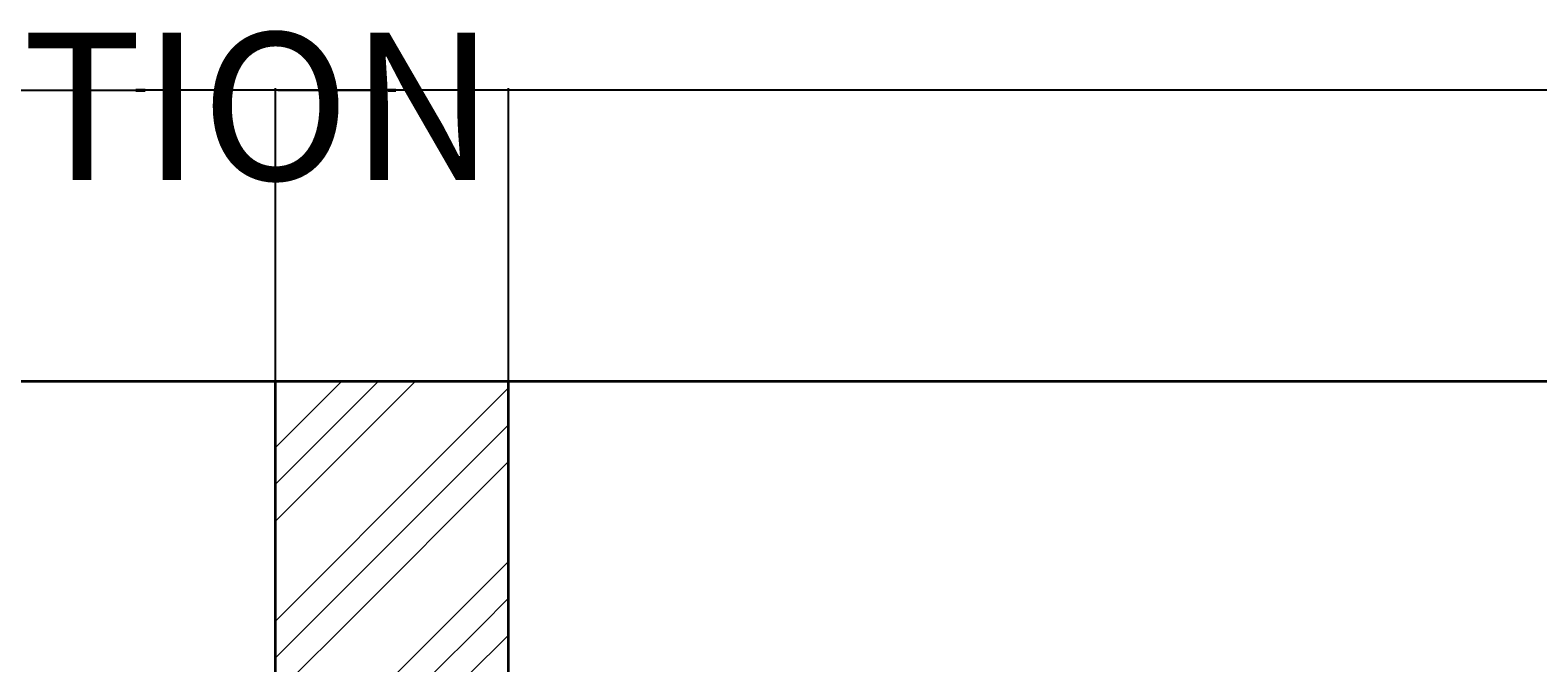
# Model space of a CAD drawing. Units: inches. Extents: x -128 to 854, y -395 to 398.
# Tile 20 of 61: x 122 to 245, y -201 to -149. Entities that reach past the tile are written whole.
import ezdxf

# ---------------------------------------------------------------- set-up
doc = ezdxf.new("R2010")
doc.units = ezdxf.units.IN
doc.header["$MEASUREMENT"] = 0
for name, color, linetype, lineweight in [('A-ANNO-DIMS', 2, 'Continuous', 18), ('A-ANNO-TITL', 7, 'Continuous', 25), ('A-SECT', 220, 'Continuous', 35), ('A-SECT-PATT', 8, 'Continuous', 13)]:
    doc.layers.add(name, color=color, linetype=linetype, lineweight=lineweight)
doc.styles.get("Standard").update_dxf_attribs({"font": 'arial.ttf'})
doc.dimstyles.get("Standard").update_dxf_attribs({"dimtxt": 0.18, "dimasz": 0.18, "dimexe": 0.18, "dimexo": 0.0625, "dimgap": 0.09, "dimtad": 0, "dimtih": 1, "dimtoh": 1, "dimdec": 1, "dimzin": 0, "dimdsep": 46, "dimlunit": 4, "dimtxsty": 'Standard', "dimcen": 0.09, "dimclrd": 1, "dimclre": 2, "dimclrt": 6, "dimadec": 0, "dimazin": 0, "dimtfac": 1, "dimtdec": 1, "dimtofl": 0, "dimtmove": 0, "dimatfit": 3, "dimfxl": 1, "dimtfill": 2, "dimtfillclr": 3, "dimtolj": 1, "dimtzin": 0, "dimarcsym": 0})

# ---------------------------------------------------------------- blocks, each defined once
blk = doc.blocks.new('*D119')
at = {"layer": 'A-ANNO-DIMS', "color": 2, "lineweight": -2, "transparency": 16777216}
for p, q in [((-56.16, -177.96), (-56.16, -154.14)), ((317.84, -177.96), (317.84, -154.14))]:
    blk.add_line(p, q, dxfattribs=at)
at = {"layer": 'A-ANNO-DIMS', "color": 1, "lineweight": -2, "transparency": 16777216}
for p, q in [((-55.98, -154.32), (130.44, -154.32)), ((317.66, -154.32), (131.24, -154.32))]:
    blk.add_line(p, q, dxfattribs=at)
at = {"layer": 'A-ANNO-DIMS', "color": 1, "transparency": 16777216}
for points in [[(-55.98, -154.29), (-55.98, -154.35), (-56.16, -154.32)], [(317.66, -154.29), (317.66, -154.35), (317.84, -154.32)]]:
    blk.add_solid(points, dxfattribs=at)
at = {"layer": 'Defpoints', "color": 0, "transparency": 16777216}
for p in [(317.84, -154.32), (-56.16, -178.02), (317.84, -178.02)]:
    blk.add_point(p, dxfattribs=at)
at = {"layer": 'A-ANNO-DIMS', "color": 6, "transparency": 16777216, "insert": (130.84, -154.32), "char_height": 0.18, "attachment_point": 5, "bg_fill": 1, "box_fill_scale": 1.25, "bg_fill_color": 3, "bg_fill_transparency": 0}
blk.add_mtext('\\A1;31\'-2"', dxfattribs=at)
blk = doc.blocks.new('*D126')
at = {"layer": 'A-ANNO-DIMS', "color": 2, "lineweight": -2, "transparency": 16777216}
for p, q in [((160.84, -178.08), (160.84, -381.9)), ((198.84, -202.08), (198.84, -381.9))]:
    blk.add_line(p, q, dxfattribs=at)
at = {"layer": 'A-ANNO-DIMS', "color": 1, "lineweight": -2, "transparency": 16777216}
for p, q in [((161.02, -381.72), (179.51, -381.72)), ((198.66, -381.72), (180.17, -381.72))]:
    blk.add_line(p, q, dxfattribs=at)
at = {"layer": 'A-ANNO-DIMS', "color": 1, "transparency": 16777216}
for points in [[(161.02, -381.69), (161.02, -381.75), (160.84, -381.72)], [(198.66, -381.69), (198.66, -381.75), (198.84, -381.72)]]:
    blk.add_solid(points, dxfattribs=at)
at = {"layer": 'Defpoints', "color": 0, "transparency": 16777216}
for p in [(160.84, -178.02), (198.84, -202.02), (198.84, -381.72)]:
    blk.add_point(p, dxfattribs=at)
at = {"layer": 'A-ANNO-DIMS', "color": 6, "transparency": 16777216, "insert": (179.84, -381.72), "char_height": 0.18, "attachment_point": 5, "bg_fill": 1, "box_fill_scale": 1.25, "bg_fill_color": 3, "bg_fill_transparency": 0}
blk.add_mtext('\\A1;3\'-2"', dxfattribs=at)
blk = doc.blocks.new('*D131')
at = {"layer": 'A-ANNO-DIMS', "color": 2, "lineweight": -2, "transparency": 16777216}
for p, q in [((141.84, -177.96), (141.84, -154.14)), ((160.84, -177.96), (160.84, -154.14))]:
    blk.add_line(p, q, dxfattribs=at)
at = {"layer": 'A-ANNO-DIMS', "color": 1, "lineweight": -2, "transparency": 16777216}
for p, q in [((142.02, -154.32), (151.02, -154.32)), ((160.66, -154.32), (151.66, -154.32))]:
    blk.add_line(p, q, dxfattribs=at)
at = {"layer": 'A-ANNO-DIMS', "color": 1, "transparency": 16777216}
for points in [[(142.02, -154.29), (142.02, -154.35), (141.84, -154.32)], [(160.66, -154.29), (160.66, -154.35), (160.84, -154.32)]]:
    blk.add_solid(points, dxfattribs=at)
at = {"layer": 'Defpoints', "color": 0, "transparency": 16777216}
for p in [(160.84, -154.32), (141.84, -178.02), (160.84, -178.02)]:
    blk.add_point(p, dxfattribs=at)
at = {"layer": 'A-ANNO-DIMS', "color": 6, "transparency": 16777216, "insert": (151.34, -154.32), "char_height": 0.18, "attachment_point": 5, "bg_fill": 1, "box_fill_scale": 1.25, "bg_fill_color": 3, "bg_fill_transparency": 0}
blk.add_mtext('\\A1;1\'-7"', dxfattribs=at)

msp = doc.modelspace()

# ---------------------------------------------------------------- hatches: boundary and pattern name
at = {"layer": 'A-SECT-PATT'}
h = msp.add_hatch(dxfattribs=at)
h.set_pattern_fill('GOST_GROUND', color=256)
h.set_pattern_definition([(45, (0, 0), (14.14214, -9e-16), [20]), (45, (3, 0), (14.14214, -9e-16), [20]), (45, (6, 0), (14.14214, -9e-16), [20])])
h.paths.add_polyline_path([(-37.16, -178.02), (-56.16, -178.02), (-56.16, -202.02), (-37.16, -202.02)])
h.paths.add_polyline_path([(160.84, -178.02), (141.84, -178.02), (141.84, -202.02), (160.84, -202.02)])
h.paths.add_polyline_path([(160.84, -207.02), (141.84, -207.02), (141.84, -226.02), (160.84, -226.02)])
h.paths.add_polyline_path([(317.84, -178.02), (298.84, -178.02), (298.84, -202.02), (317.84, -202.02)])
h.paths.add_polyline_path([(317.84, -207.02), (298.84, -207.02), (298.84, -226.02), (317.84, -226.02)])
h.paths.add_polyline_path([(317.84, -274.02), (298.84, -274.02), (298.84, -298.02), (303.84, -298.02), (312.84, -298.02), (317.84, -298.02)])

# ---------------------------------------------------------------- linework, layer by layer
at = {"layer": 'A-SECT'}
for p, q in [((-56.16, -178.02), (317.84, -178.02)), ((141.84, -298.02), (141.84, -178.02)), ((160.84, -298.02), (160.84, -178.02))]:
    msp.add_line(p, q, dxfattribs=at)

# ---------------------------------------------------------------- texts
at = {"layer": 'A-ANNO-TITL'}
msp.add_text('SECTION', height=12, dxfattribs=at).set_placement((91.33, -161.64))

# ---------------------------------------------------------------- dimensions: what is measured, and where the dimension line sits
at = {"layer": 'A-ANNO-DIMS'}
for base, p1, p2, picture, middle in [((317.84, -154.32), (-56.16, -178.02), (317.84, -178.02), '*D119', (130.84, -154.32)), ((160.84, -154.32), (141.84, -178.02), (160.84, -178.02), '*D131', (151.34, -154.32)), ((198.84, -381.72), (160.84, -178.02), (198.84, -202.02), '*D126', (179.84, -381.72))]:
    dim = msp.add_linear_dim(base=base, p1=p1, p2=p2, dimstyle='Standard', override={"dimdec": 1, "dimlfac": 1, "dimrnd": 0, "dimzin": 1, "dimdsep": 46, "dimlunit": 4, "dimfrac": 2}, dxfattribs=at)
    dim.commit()
    dim.dimension.update_dxf_attribs({"geometry": picture, "text_midpoint": middle})

doc.saveas('drawing.dxf')
